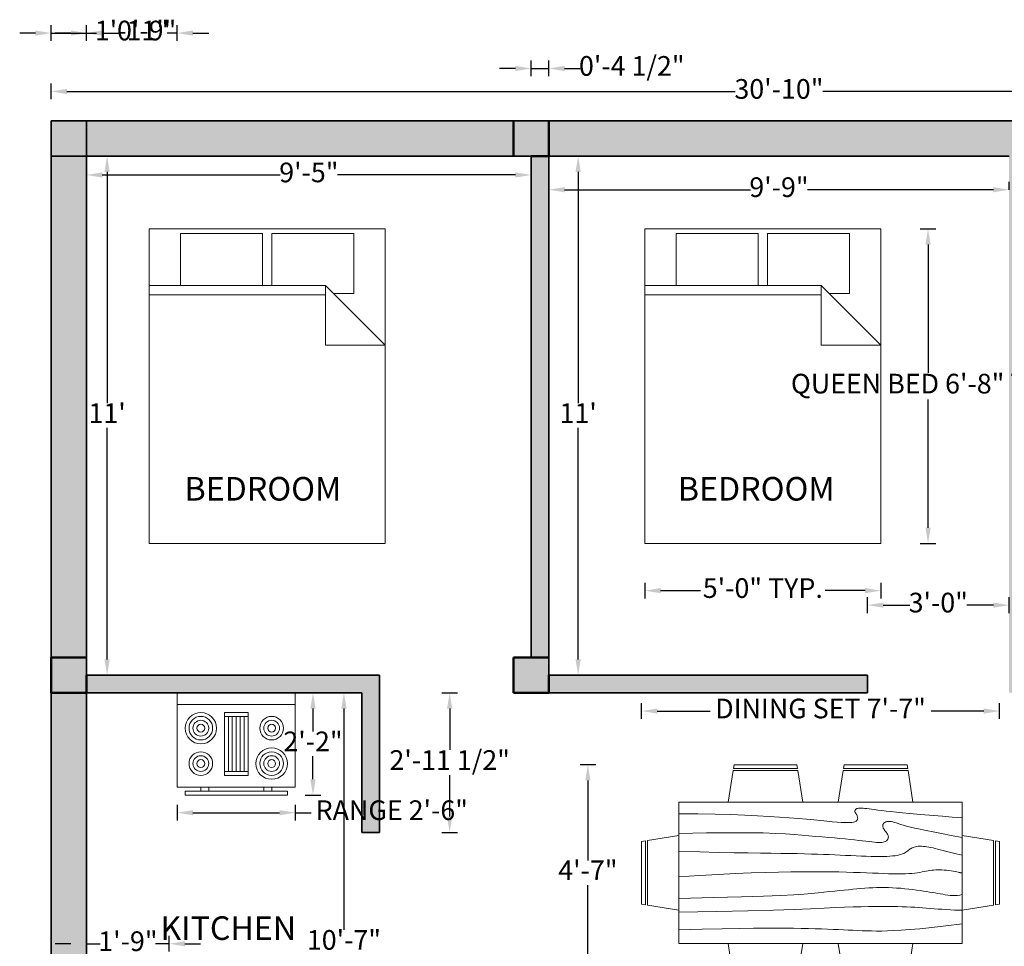
# Model space of a CAD drawing. Units: inches. Extents: x 2244 to 2676, y 593 to 1067.
# Tile 3 of 4: x 2268 to 2518, y 831 to 1067. Entities that reach past the tile are written whole.
import ezdxf

# ---------------------------------------------------------------- set-up
doc = ezdxf.new("R2010")
doc.units = ezdxf.units.IN
for name, color, linetype, lineweight in [('A-ANNO-DIMS', 2, 'Continuous', 18), ('A-AREA-IDEN', 7, 'Continuous', 25), ('A-COLS', 7, 'Continuous', 50), ('A-COLS-PATT', 1, 'Continuous', 13), ('A-EQPM', 8, 'Continuous', 18), ('A-FURN', 8, 'Continuous', 18), ('A-WALL', 7, 'Continuous', 35)]:
    doc.layers.add(name, color=color, linetype=linetype, lineweight=lineweight)
doc.layers.add('A-WALL-PATT', color=159, linetype='Continuous', lineweight=13, true_color=0x22346e)
doc.styles.get("Standard").update_dxf_attribs({"font": 'arial.ttf'})
doc.dimstyles.new('ISO-25', dxfattribs={"dimtxt": 5, "dimasz": 4, "dimexe": 2, "dimexo": 2, "dimtad": 0, "dimtih": 1, "dimtoh": 1, "dimlunit": 3, "dimtxsty": 'Standard', "dimcen": 2.5, "dimadec": 0, "dimazin": 0, "dimtfac": 1, "dimtmove": 0, "dimatfit": 3, "dimfxl": 2, "dimfxlon": 1, "dimarcsym": 0})

# ---------------------------------------------------------------- blocks, each defined once
blk = doc.blocks.new('*D4')
at = {"layer": 'A-ANNO-DIMS', "color": 0, "lineweight": -2, "transparency": 16777216}
for p, q in [((2288.42, 1031.92), (2292.42, 1031.92)), ((2290.42, 1027.92), (2290.42, 969.06)), ((2290.42, 903.92), (2290.42, 962.79)), ((2288.42, 899.92), (2292.42, 899.92))]:
    blk.add_line(p, q, dxfattribs=at)
at = {"layer": 'A-ANNO-DIMS', "color": 0, "transparency": 16777216}
for points in [[(2289.75, 1027.92), (2291.08, 1027.92), (2290.42, 1031.92)], [(2289.75, 903.92), (2291.08, 903.92), (2290.42, 899.92)]]:
    blk.add_solid(points, dxfattribs=at)
at = {"layer": 'Defpoints', "color": 0, "transparency": 16777216}
for p in [(2285.2, 1031.92), (2285.2, 899.92), (2290.42, 899.92)]:
    blk.add_point(p, dxfattribs=at)
at = {"layer": 'A-ANNO-DIMS', "color": 0, "transparency": 16777216, "insert": (2290.42, 965.92), "char_height": 5, "attachment_point": 5}
blk.add_mtext("11'", dxfattribs=at)
blk = doc.blocks.new('*D5')
at = {"layer": 'A-ANNO-DIMS', "color": 0, "lineweight": -2, "transparency": 16777216}
for p, q in [((2285.2, 1025.13), (2285.2, 1029.13)), ((2398.2, 1025.13), (2398.2, 1029.13)), ((2289.2, 1027.13), (2334.43, 1027.13)), ((2394.2, 1027.13), (2348.97, 1027.13))]:
    blk.add_line(p, q, dxfattribs=at)
at = {"layer": 'A-ANNO-DIMS', "color": 0, "transparency": 16777216}
for points in [[(2289.2, 1027.8), (2289.2, 1026.47), (2285.2, 1027.13)], [(2394.2, 1027.8), (2394.2, 1026.47), (2398.2, 1027.13)]]:
    blk.add_solid(points, dxfattribs=at)
at = {"layer": 'Defpoints', "color": 0, "transparency": 16777216}
for p in [(2398.2, 1027.13), (2285.2, 1019.69), (2398.2, 1019.69)]:
    blk.add_point(p, dxfattribs=at)
at = {"layer": 'A-ANNO-DIMS', "color": 0, "transparency": 16777216, "insert": (2341.7, 1027.13), "char_height": 5, "attachment_point": 5}
blk.add_mtext('9\'-5"', dxfattribs=at)
blk = doc.blocks.new('*D6')
at = {"layer": 'A-ANNO-DIMS', "color": 0, "lineweight": -2, "transparency": 16777216}
for p, q in [((2402.7, 1023.38), (2402.7, 1025.38)), ((2519.7, 1023.38), (2519.7, 1025.38)), ((2406.7, 1023.38), (2453.93, 1023.38)), ((2515.7, 1023.38), (2468.47, 1023.38))]:
    blk.add_line(p, q, dxfattribs=at)
at = {"layer": 'A-ANNO-DIMS', "color": 0, "transparency": 16777216}
for points in [[(2406.7, 1024.05), (2406.7, 1022.72), (2402.7, 1023.38)], [(2515.7, 1024.05), (2515.7, 1022.72), (2519.7, 1023.38)]]:
    blk.add_solid(points, dxfattribs=at)
at = {"layer": 'Defpoints', "color": 0, "transparency": 16777216}
for p in [(2402.7, 1023.38), (2402.7, 1022.02), (2519.7, 1022.02)]:
    blk.add_point(p, dxfattribs=at)
at = {"layer": 'A-ANNO-DIMS', "color": 0, "transparency": 16777216, "insert": (2461.2, 1023.38), "char_height": 5, "attachment_point": 5}
blk.add_mtext('9\'-9"', dxfattribs=at)
blk = doc.blocks.new('*D7')
at = {"layer": 'A-ANNO-DIMS', "color": 0, "lineweight": -2, "transparency": 16777216}
for p, q in [((2412.16, 1031.92), (2408.16, 1031.92)), ((2410.16, 1027.92), (2410.16, 969.06)), ((2410.16, 903.92), (2410.16, 962.79)), ((2412.16, 899.92), (2408.16, 899.92))]:
    blk.add_line(p, q, dxfattribs=at)
at = {"layer": 'A-ANNO-DIMS', "color": 0, "transparency": 16777216}
for points in [[(2409.49, 1027.92), (2410.82, 1027.92), (2410.16, 1031.92)], [(2409.49, 903.92), (2410.82, 903.92), (2410.16, 899.92)]]:
    blk.add_solid(points, dxfattribs=at)
at = {"layer": 'Defpoints', "color": 0, "transparency": 16777216}
for p in [(2414.35, 1031.92), (2410.16, 899.92), (2414.35, 899.92)]:
    blk.add_point(p, dxfattribs=at)
at = {"layer": 'A-ANNO-DIMS', "color": 0, "transparency": 16777216, "insert": (2410.16, 965.92), "char_height": 5, "attachment_point": 5}
blk.add_mtext("11'", dxfattribs=at)
blk = doc.blocks.new('*D21')
at = {"layer": 'A-ANNO-DIMS', "color": 0, "lineweight": -2, "transparency": 16777216}
for p, q in [((2276.2, 1046.37), (2276.2, 1050.37)), ((2646.2, 1046.37), (2646.2, 1050.37)), ((2280.2, 1048.37), (2450.04, 1048.37)), ((2642.2, 1048.37), (2472.35, 1048.37))]:
    blk.add_line(p, q, dxfattribs=at)
at = {"layer": 'A-ANNO-DIMS', "color": 0, "transparency": 16777216}
for points in [[(2280.2, 1049.03), (2280.2, 1047.7), (2276.2, 1048.37)], [(2642.2, 1049.03), (2642.2, 1047.7), (2646.2, 1048.37)]]:
    blk.add_solid(points, dxfattribs=at)
at = {"layer": 'Defpoints', "color": 0, "transparency": 16777216}
for p in [(2646.2, 1048.37), (2276.2, 1040.92), (2646.2, 1040.92)]:
    blk.add_point(p, dxfattribs=at)
at = {"layer": 'A-ANNO-DIMS', "color": 0, "transparency": 16777216, "insert": (2461.2, 1048.37), "char_height": 5, "attachment_point": 5}
blk.add_mtext('30\'-10"', dxfattribs=at)
blk = doc.blocks.new('Dining Set - 36 x 72 in.')
for p, q in [((-22.2343, 26.00059), (-23.4847, 17.99762)), ((-22.2304, 26), (-5.7608, 26)), ((-22, 27.5), (-22.1562, 26.50042)), ((-5.8416, 26.5), (-22.1534, 26.5)), ((-22, 27.5), (-6, 27.5)), ((-5.8437, 26.49966), (-6, 27.5)), ((-4.5152, 17.99762), (-5.7655, 25.99926)), ((5.7657, 26.00059), (4.5153, 17.99762)), ((5.7696, 26), (22.2392, 26)), ((6, 27.5), (5.8438, 26.50042)), ((22.1584, 26.5), (5.8466, 26.5)), ((6, 27.5), (22, 27.5)), ((22.1563, 26.49966), (22, 27.5)), ((23.4848, 17.99762), (22.2345, 25.99926)), ((36, 18), (-36, 18)), ((-36, 18), (-36, -18)), ((36, -18), (36, 18)), ((-45.5, 8), (-44.5004, 8.15617)), ((-45.5, 8), (-45.5, -8)), ((-44.5, -8.15843), (-44.5, 8.15338)), ((-44.0006, 8.23428), (-35.9976, 9.48474)), ((-44, 8.23041), (-44, -8.23915)), ((44.0006, 8.23428), (35.9976, 9.48474)), ((44, 8.23041), (44, -8.23915)), ((44.5, -8.15843), (44.5, 8.15338)), ((45.5, 8), (44.5005, 8.15617)), ((45.5, 8), (45.5, -8)), ((-44.4997, -8.15631), (-45.5, -8)), ((-35.9976, -9.48476), (-43.9993, -8.2345)), ((35.9976, -9.48476), (43.9993, -8.2345)), ((44.4997, -8.15631), (45.5, -8)), ((-36, -18), (36, -18)), ((-22.2343, -26.0006), (-23.4847, -17.99762)), ((-4.5152, -17.99762), (-5.7655, -25.99928)), ((5.7657, -26.0006), (4.5153, -17.99762)), ((23.4848, -17.99762), (22.2345, -25.99928)), ((-22.2304, -26), (-5.7608, -26)), ((-22, -27.5), (-22.1562, -26.50044)), ((-5.8416, -26.5), (-22.1534, -26.5)), ((-22, -27.5), (-6, -27.5)), ((-5.8437, -26.49967), (-6, -27.5)), ((5.7696, -26), (22.2392, -26)), ((6, -27.5), (5.8438, -26.50044)), ((22.1584, -26.5), (5.8466, -26.5)), ((6, -27.5), (22, -27.5)), ((22.1563, -26.49967), (22, -27.5))]:
    blk.add_line(p, q)
for points in [[(-36, 15), (-31.1772, 14.97754), (-26.8079, 14.91406), (-22.8538, 14.81543), (-19.276, 14.6875), (-16.0362, 14.53613), (-13.0957, 14.36718), (-10.4159, 14.18652), (-7.9583, 14), (-5.6904, 13.81315), (-3.6035, 13.63021), (-1.6954, 13.45508), (0.0365, 13.29166), (1.5945, 13.14388), (2.9811, 13.01562), (4.1988, 12.9108), (5.25, 12.83333), (6.1393, 12.78613), (6.8802, 12.76823), (7.4883, 12.77767), (7.9792, 12.8125), (8.3685, 12.87077), (8.6719, 12.95052), (8.9049, 13.0498), (9.0833, 13.16666), (9.2205, 13.29899), (9.3216, 13.44401), (9.3895, 13.59879), (9.4271, 13.76041), (9.4373, 13.92594), (9.4232, 14.09245), (9.3875, 14.257), (9.3333, 14.41666), (9.2638, 14.56917), (9.1836, 14.71484), (9.0975, 14.85465), (9.0104, 14.98958), (8.9272, 15.1206), (8.8529, 15.2487), (8.7922, 15.37483), (8.75, 15.5), (8.7305, 15.62467), (8.7344, 15.74739), (8.7617, 15.86621), (8.8125, 15.97916), (8.8867, 16.08431), (8.9844, 16.17968), (9.1055, 16.26334), (9.25, 16.33333), (9.4189, 16.38802), (9.6172, 16.42708), (9.8506, 16.45052), (10.125, 16.45833), (10.4463, 16.45052), (10.8203, 16.42708), (11.2529, 16.38802), (11.75, 16.33333), (12.3184, 16.26318), (12.9694, 16.17838), (13.7151, 16.07991), (14.5677, 15.96875), (15.5395, 15.84586), (16.6426, 15.71224), (17.8893, 15.56884), (19.2917, 15.41666), (20.859, 15.25667), (22.5879, 15.08984), (24.4721, 14.91715), (26.5052, 14.73958), (28.6809, 14.5581), (30.9929, 14.3737), (33.4347, 14.18733), (36, 14)], [(-36, 10), (-28.9766, 10.14274), (-23.1725, 10.20442), (-18.4241, 10.19775), (-14.5677, 10.13541), (-11.4399, 10.03011), (-8.877, 9.89453), (-6.7154, 9.74137), (-4.7917, 9.58333), (-2.9698, 9.43082), (-1.2246, 9.28515), (0.4415, 9.14534), (2.026, 9.01041), (3.5266, 8.87939), (4.9408, 8.7513), (6.266, 8.62516), (7.5, 8.5), (8.6411, 8.37549), (9.6914, 8.2539), (10.6538, 8.13818), (11.5312, 8.03125), (12.3267, 7.93603), (13.043, 7.85547), (13.6831, 7.79248), (14.25, 7.75), (14.7471, 7.7303), (15.1797, 7.73307), (15.5537, 7.75732), (15.875, 7.80208), (16.1494, 7.86637), (16.3828, 7.94922), (16.5811, 8.04964), (16.75, 8.16666), (16.8944, 8.29915), (17.0143, 8.44531), (17.1089, 8.60319), (17.1771, 8.77083), (17.218, 8.94629), (17.2305, 9.1276), (17.2137, 9.31282), (17.1667, 9.5), (17.0895, 9.6875), (16.987, 9.875), (16.8649, 10.0625), (16.7292, 10.25), (16.5856, 10.4375), (16.4401, 10.625), (16.2985, 10.8125), (16.1667, 11), (16.05, 11.18733), (15.9518, 11.3737), (15.8752, 11.5581), (15.8229, 11.73958), (15.798, 11.91715), (15.8034, 12.08984), (15.842, 12.25667), (15.9167, 12.41666), (16.0295, 12.56836), (16.1784, 12.70833), (16.3605, 12.83268), (16.5729, 12.9375), (16.8127, 13.01888), (17.0768, 13.07291), (17.3625, 13.0957), (17.6667, 13.08333), (17.9894, 13.03312), (18.3418, 12.94726), (18.7382, 12.82918), (19.1927, 12.68229), (19.7195, 12.51001), (20.3327, 12.31575), (21.0465, 12.10294), (21.875, 11.875), (22.8357, 11.63354), (23.959, 11.37304), (25.2786, 11.08618), (26.8282, 10.76562), (28.6414, 10.40405), (30.752, 9.99414), (33.1936, 9.52856), (36, 9)], [(-36, 5.5), (-30.7157, 5.3348), (-26.069, 5.20963), (-21.9946, 5.11767), (-18.4271, 5.05208), (-15.3009, 5.00602), (-12.5508, 4.97265), (-10.1112, 4.94515), (-7.9167, 4.91666), (-5.909, 4.88167), (-4.0586, 4.83984), (-2.3429, 4.79215), (-0.7396, 4.73958), (0.7739, 4.6831), (2.22, 4.6237), (3.6213, 4.56233), (5, 4.5), (6.373, 4.43782), (7.7344, 4.3776), (9.0723, 4.32129), (10.375, 4.27083), (11.6309, 4.22819), (12.8281, 4.19531), (13.9551, 4.17415), (15, 4.16666), (15.954, 4.17448), (16.819, 4.19791), (17.6001, 4.23698), (18.3021, 4.29166), (18.9299, 4.36198), (19.4883, 4.44791), (19.9823, 4.54948), (20.4167, 4.66666), (20.7969, 4.79899), (21.1302, 4.94401), (21.4245, 5.09879), (21.6875, 5.26041), (21.9271, 5.42594), (22.1511, 5.59245), (22.3672, 5.757), (22.5834, 5.91666), (22.8065, 6.06868), (23.0404, 6.21093), (23.2879, 6.34147), (23.5521, 6.45833), (23.8358, 6.55957), (24.142, 6.64323), (24.4735, 6.70735), (24.8334, 6.75), (25.2235, 6.76969), (25.642, 6.76692), (26.0858, 6.74267), (26.5521, 6.69791), (27.0379, 6.63362), (27.5404, 6.55078), (28.0565, 6.45036), (28.5834, 6.33333), (29.1242, 6.19987), (29.7071, 6.04687), (30.3661, 5.87044), (31.1354, 5.66666), (32.0493, 5.43164), (33.142, 5.16146), (34.4475, 4.85221), (36, 4.5)], [(-36, -1), (-30.7915, -0.6591), (-26.0195, -0.38216), (-21.6519, -0.16284), (-17.6563, 0.00521), (-14.0005, 0.12833), (-10.6523, 0.21289), (-7.5796, 0.26522), (-4.75, 0.29166), (-2.134, 0.29793), (0.2878, 0.28711), (2.5317, 0.26163), (4.6146, 0.22396), (6.5529, 0.17651), (8.3633, 0.12174), (10.0623, 0.06209), (11.6667, 0), (13.1899, -0.06201), (14.6341, -0.1211), (15.9982, -0.17432), (17.2813, -0.21875), (18.4823, -0.25147), (19.6003, -0.26953), (20.6343, -0.27002), (21.5834, -0.25), (22.4481, -0.20768), (23.2357, -0.14584), (23.9549, -0.06836), (24.6146, 0.02083), (25.2235, 0.11784), (25.7904, 0.21875), (26.3241, 0.31966), (26.8334, 0.41666), (27.3265, 0.50618), (27.8099, 0.58593), (28.2894, 0.65397), (28.7709, 0.70833), (29.2601, 0.74707), (29.763, 0.76823), (30.2855, 0.76985), (30.8334, 0.75), (31.4088, 0.70784), (31.9994, 0.64713), (32.589, 0.57275), (33.1615, 0.48958), (33.7008, 0.4025), (34.1908, 0.3164), (34.6153, 0.23616), (34.9584, 0.16666), (35.2099, 0.11165), (35.3848, 0.07031), (35.504, 0.04069), (35.5886, 0.02083), (35.6594, 0.00879), (35.7377, 0.0026), (35.8442, 0.00032), (36, 0)], [(-36, -6.5), (-27.1843, -6.31267), (-20.084, -6.1263), (-14.469, -5.9419), (-10.1094, -5.76042), (-6.7752, -5.58285), (-4.2363, -5.41016), (-2.2629, -5.24333), (-0.625, -5.08334), (0.8708, -4.93099), (2.2715, -4.78646), (3.5872, -4.64974), (4.8281, -4.52084), (6.0046, -4.39974), (7.127, -4.28646), (8.2053, -4.18099), (9.25, -4.08334), (10.2705, -3.99382), (11.2734, -3.91407), (12.2647, -3.84603), (13.25, -3.79167), (14.2354, -3.75293), (15.2266, -3.73177), (16.2295, -3.73015), (17.25, -3.75), (18.2912, -3.79248), (19.3451, -3.85547), (20.4009, -3.93604), (21.4479, -4.03125), (22.4754, -4.13819), (23.4727, -4.25391), (24.4289, -4.37549), (25.3334, -4.5), (26.1785, -4.62492), (26.9694, -4.74935), (27.7145, -4.87281), (28.4219, -4.99479), (29.1, -5.11483), (29.7572, -5.23242), (30.4016, -5.34709), (31.0417, -5.45834), (31.6837, -5.56437), (32.3262, -5.65821), (32.9658, -5.73153), (33.599, -5.77604), (34.2224, -5.78345), (34.8327, -5.74545), (35.4264, -5.65373), (36, -5.5)], [(-36, -10), (-26.4022, -9.81299), (-18.4675, -9.62891), (-11.9839, -9.45069), (-6.7396, -9.28125), (-2.5226, -9.12354), (0.8789, -8.98047), (3.6769, -8.85498), (6.0833, -8.75), (8.2767, -8.66765), (10.3021, -8.60677), (12.1712, -8.56543), (13.8958, -8.54167), (15.4876, -8.53353), (16.9583, -8.53907), (18.3197, -8.55632), (19.5834, -8.58334), (20.7616, -8.61841), (21.8685, -8.66081), (22.9188, -8.71004), (23.9271, -8.76563), (24.9081, -8.82707), (25.8763, -8.89388), (26.8465, -8.96558), (27.8334, -9.04167), (28.8474, -9.12118), (29.8828, -9.20117), (30.93, -9.27824), (31.9792, -9.34896), (33.0205, -9.40991), (34.0443, -9.45768), (35.0407, -9.48885), (36, -9.5)], [(-36, -14.5), (-30.0881, -14.33513), (-25.0332, -14.21224), (-20.7312, -14.12647), (-17.0781, -14.07292), (-13.97, -14.04671), (-11.3027, -14.04297), (-8.9724, -14.05681), (-6.875, -14.08334), (-4.9224, -14.11833), (-3.0905, -14.16016), (-1.3709, -14.20785), (0.2448, -14.26042), (1.7647, -14.3169), (3.1973, -14.3763), (4.5507, -14.43767), (5.8333, -14.5), (7.0554, -14.5621), (8.235, -14.62175), (9.3922, -14.67652), (10.5469, -14.72396), (11.7192, -14.76164), (12.929, -14.78711), (14.1965, -14.79794), (15.5417, -14.79167), (16.9933, -14.76424), (18.6152, -14.70508), (20.4804, -14.60197), (22.6615, -14.44271), (25.2312, -14.21509), (28.2624, -13.9069), (31.8277, -13.50594), (36, -13)]]:
    blk.add_lwpolyline(points)
blk = doc.blocks.new('Range-Oven - 30 in top')
for p, q in [((0, -3), (30, -3)), ((12, -6), (18, -6)), ((13, -20), (13, -6)), ((14, -6), (14, -20)), ((15, -20), (15, -6)), ((16, -6), (16, -20)), ((17, -20), (17, -6)), ((18, -20), (12, -20)), ((6, -24), (6, -25)), ((8, -25), (8, -24)), ((22, -25), (22, -24)), ((24, -24), (24, -25))]:
    blk.add_line(p, q)
for points in [[(0, -24), (0, 0), (30, 0), (30, -24)], [(12, -21), (12, -5), (18, -5), (18, -21)], [(2, -26), (2, -25), (28, -25), (28, -26)]]:
    blk.add_lwpolyline(points, close=True)
for centre, radius in [((6, -9), 4), ((6, -9), 3), ((6, -9), 2), ((24, -9), 3), ((24, -9), 2), ((6, -9), 1), ((24, -9), 1), ((6, -18), 3), ((24, -18), 4), ((24, -18), 3), ((6, -18), 2), ((6, -18), 1), ((24, -18), 2), ((24, -18), 1)]:
    blk.add_circle(centre, radius)
blk = doc.blocks.new('Bed - Queen')
for p, q in [((0, -80.00003), (0, 0)), ((0, 0), (59.99999, 0)), ((59.99999, 0), (59.99999, -80.00003)), ((7.99999, -1.2), (28.79998, -1.2)), ((7.99999, -14.4), (7.99999, -1.2)), ((28.79998, -1.2), (28.79998, -14.4)), ((31.19999, -1.2), (51.99999, -1.2)), ((31.19999, -14.4), (31.19999, -1.2)), ((51.99999, -1.2), (51.99999, -16.4)), ((0, -14.4), (44.8, -14.4)), ((59.99999, -29.6), (44.8, -14.4)), ((44.8, -14.4), (44.8, -29.6)), ((44.8, -16.8), (0, -16.8)), ((51.99999, -16.4), (46.79936, -16.4)), ((44.8, -29.6), (59.99999, -29.6)), ((59.99999, -80.00003), (0, -80.00003))]:
    blk.add_line(p, q)
blk = doc.blocks.new('*D28')
at = {"layer": 'A-ANNO-DIMS', "color": 0, "lineweight": -2, "transparency": 16777216}
for p, q in [((2352.62, 895.42), (2348.62, 895.42)), ((2350.62, 891.42), (2350.62, 835.1)), ((2350.62, 772.42), (2350.62, 828.74)), ((2352.62, 768.42), (2348.62, 768.42))]:
    blk.add_line(p, q, dxfattribs=at)
at = {"layer": 'A-ANNO-DIMS', "color": 0, "transparency": 16777216}
for points in [[(2349.96, 891.42), (2351.29, 891.42), (2350.62, 895.42)], [(2349.96, 772.42), (2351.29, 772.42), (2350.62, 768.42)]]:
    blk.add_solid(points, dxfattribs=at)
at = {"layer": 'Defpoints', "color": 0, "transparency": 16777216}
for p in [(2355.2, 895.42), (2350.62, 768.42), (2355.2, 768.42)]:
    blk.add_point(p, dxfattribs=at)
at = {"layer": 'A-ANNO-DIMS', "color": 0, "transparency": 16777216, "insert": (2350.62, 831.92), "char_height": 5, "attachment_point": 5}
blk.add_mtext('10\'-7"', dxfattribs=at)
blk = doc.blocks.new('*D30')
at = {"layer": 'A-ANNO-DIMS', "color": 0, "lineweight": -2, "transparency": 16777216}
for p, q in [((2497.1, 1013.41), (2501.1, 1013.41)), ((2499.1, 1009.41), (2499.1, 976.77)), ((2499.1, 937.41), (2499.1, 970.04)), ((2497.1, 933.41), (2501.1, 933.41))]:
    blk.add_line(p, q, dxfattribs=at)
at = {"layer": 'A-ANNO-DIMS', "color": 0, "transparency": 16777216}
for points in [[(2498.44, 1009.41), (2499.77, 1009.41), (2499.1, 1013.41)], [(2498.44, 937.41), (2499.77, 937.41), (2499.1, 933.41)]]:
    blk.add_solid(points, dxfattribs=at)
at = {"layer": 'Defpoints', "color": 0, "transparency": 16777216}
for p in [(2487.1, 1013.41), (2499.1, 1013.41), (2487.1, 933.41)]:
    blk.add_point(p, dxfattribs=at)
at = {"layer": 'A-ANNO-DIMS', "color": 0, "transparency": 16777216, "insert": (2499.1, 973.41), "char_height": 5, "attachment_point": 5}
blk.add_mtext('QUEEN BED 6\'-8" TYP.', dxfattribs=at)
blk = doc.blocks.new('*D31')
at = {"layer": 'A-ANNO-DIMS', "color": 0, "lineweight": -2, "transparency": 16777216}
for p, q in [((2427.1, 923.41), (2427.1, 919.41)), ((2431.1, 921.41), (2441.24, 921.41)), ((2483.1, 921.41), (2472.97, 921.41)), ((2487.1, 923.41), (2487.1, 919.41))]:
    blk.add_line(p, q, dxfattribs=at)
at = {"layer": 'A-ANNO-DIMS', "color": 0, "transparency": 16777216}
for points in [[(2431.1, 922.07), (2431.1, 920.74), (2427.1, 921.41)], [(2483.1, 922.07), (2483.1, 920.74), (2487.1, 921.41)]]:
    blk.add_solid(points, dxfattribs=at)
at = {"layer": 'Defpoints', "color": 0, "transparency": 16777216}
for p in [(2427.1, 933.41), (2487.1, 933.41), (2487.1, 921.41)]:
    blk.add_point(p, dxfattribs=at)
at = {"layer": 'A-ANNO-DIMS', "color": 0, "transparency": 16777216, "insert": (2457.1, 921.41), "char_height": 5, "attachment_point": 5}
blk.add_mtext('5\'-0" TYP.', dxfattribs=at)
blk = doc.blocks.new('*D32')
at = {"layer": 'A-ANNO-DIMS', "color": 0, "lineweight": -2, "transparency": 16777216}
for p, q in [((2426.28, 888.78), (2426.28, 892.78)), ((2517.28, 888.78), (2517.28, 892.78)), ((2430.28, 890.78), (2443.68, 890.78)), ((2513.28, 890.78), (2499.88, 890.78))]:
    blk.add_line(p, q, dxfattribs=at)
at = {"layer": 'A-ANNO-DIMS', "color": 0, "transparency": 16777216}
for points in [[(2430.28, 891.45), (2430.28, 890.11), (2426.28, 890.78)], [(2513.28, 891.45), (2513.28, 890.11), (2517.28, 890.78)]]:
    blk.add_solid(points, dxfattribs=at)
at = {"layer": 'Defpoints', "color": 0, "transparency": 16777216}
for p in [(2517.28, 890.78), (2426.28, 877.13), (2517.28, 877.13)]:
    blk.add_point(p, dxfattribs=at)
at = {"layer": 'A-ANNO-DIMS', "color": 0, "transparency": 16777216, "insert": (2471.78, 890.78), "char_height": 5, "attachment_point": 5}
blk.add_mtext('DINING SET 7\'-7"', dxfattribs=at)
blk = doc.blocks.new('*D33')
at = {"layer": 'A-ANNO-DIMS', "color": 0, "lineweight": -2, "transparency": 16777216}
for p, q in [((2414.63, 877.13), (2410.63, 877.13)), ((2412.63, 873.13), (2412.63, 852.75)), ((2412.63, 826.13), (2412.63, 846.5)), ((2414.63, 822.13), (2410.63, 822.13))]:
    blk.add_line(p, q, dxfattribs=at)
at = {"layer": 'A-ANNO-DIMS', "color": 0, "transparency": 16777216}
for points in [[(2411.96, 873.13), (2413.3, 873.13), (2412.63, 877.13)], [(2411.96, 826.13), (2413.3, 826.13), (2412.63, 822.13)]]:
    blk.add_solid(points, dxfattribs=at)
at = {"layer": 'Defpoints', "color": 0, "transparency": 16777216}
for p in [(2412.63, 877.13), (2426.28, 877.13), (2426.28, 822.13)]:
    blk.add_point(p, dxfattribs=at)
at = {"layer": 'A-ANNO-DIMS', "color": 0, "transparency": 16777216, "insert": (2412.63, 849.63), "char_height": 5, "attachment_point": 5}
blk.add_mtext('4\'-7"', dxfattribs=at)
blk = doc.blocks.new('*D37')
at = {"layer": 'A-ANNO-DIMS', "color": 0, "lineweight": -2, "transparency": 16777216}
for p, q in [((2285.2, 829.59), (2285.2, 833.59)), ((2306.2, 829.59), (2306.2, 833.59)), ((2281.2, 831.59), (2277.2, 831.59)), ((2285.2, 831.59), (2288.66, 831.59)), ((2306.2, 831.59), (2302.73, 831.59)), ((2310.2, 831.59), (2314.2, 831.59))]:
    blk.add_line(p, q, dxfattribs=at)
at = {"layer": 'A-ANNO-DIMS', "color": 0, "transparency": 16777216}
for points in [[(2281.2, 832.25), (2281.2, 830.92), (2285.2, 831.59)], [(2310.2, 832.25), (2310.2, 830.92), (2306.2, 831.59)]]:
    blk.add_solid(points, dxfattribs=at)
at = {"layer": 'Defpoints', "color": 0, "transparency": 16777216}
for p in [(2285.2, 831.59), (2285.2, 826.19), (2306.2, 826.19)]:
    blk.add_point(p, dxfattribs=at)
at = {"layer": 'A-ANNO-DIMS', "color": 0, "transparency": 16777216, "insert": (2295.7, 831.59), "char_height": 5, "attachment_point": 5}
blk.add_mtext('1\'-9"', dxfattribs=at)
blk = doc.blocks.new('*D38')
at = {"layer": 'A-ANNO-DIMS', "color": 0, "lineweight": -2, "transparency": 16777216}
for p, q in [((2308.25, 866.92), (2308.25, 862.92)), ((2338.25, 866.92), (2338.25, 862.92)), ((2312.25, 864.92), (2334.25, 864.92)), ((2338.25, 864.92), (2342.25, 864.92))]:
    blk.add_line(p, q, dxfattribs=at)
at = {"layer": 'A-ANNO-DIMS', "color": 0, "transparency": 16777216}
for points in [[(2312.25, 865.59), (2312.25, 864.25), (2308.25, 864.92)], [(2334.25, 865.59), (2334.25, 864.25), (2338.25, 864.92)]]:
    blk.add_solid(points, dxfattribs=at)
at = {"layer": 'Defpoints', "color": 0, "transparency": 16777216}
for p in [(2308.25, 869.42), (2338.25, 869.42), (2338.25, 864.92)]:
    blk.add_point(p, dxfattribs=at)
at = {"layer": 'A-ANNO-DIMS', "color": 0, "transparency": 16777216, "insert": (2362.78, 864.92), "char_height": 5, "attachment_point": 5}
blk.add_mtext('RANGE 2\'-6"', dxfattribs=at)
blk = doc.blocks.new('*D39')
at = {"layer": 'A-ANNO-DIMS', "color": 0, "lineweight": -2, "transparency": 16777216}
for p, q in [((2340.75, 895.42), (2344.75, 895.42)), ((2342.75, 891.42), (2342.75, 885.56)), ((2342.75, 873.42), (2342.75, 879.29)), ((2340.75, 869.42), (2344.75, 869.42))]:
    blk.add_line(p, q, dxfattribs=at)
at = {"layer": 'A-ANNO-DIMS', "color": 0, "transparency": 16777216}
for points in [[(2342.08, 891.42), (2343.42, 891.42), (2342.75, 895.42)], [(2342.08, 873.42), (2343.42, 873.42), (2342.75, 869.42)]]:
    blk.add_solid(points, dxfattribs=at)
at = {"layer": 'Defpoints', "color": 0, "transparency": 16777216}
for p in [(2338.25, 895.42), (2342.75, 895.42), (2338.25, 869.42)]:
    blk.add_point(p, dxfattribs=at)
at = {"layer": 'A-ANNO-DIMS', "color": 0, "transparency": 16777216, "insert": (2342.75, 882.42), "char_height": 5, "attachment_point": 5}
blk.add_mtext('2\'-2"', dxfattribs=at)
blk = doc.blocks.new('*D42')
at = {"layer": 'A-ANNO-DIMS', "color": 0, "lineweight": -2, "transparency": 16777216}
for p, q in [((2666.5, 859.92), (2670.5, 859.92)), ((2668.5, 855.92), (2668.5, 835.1)), ((2668.5, 807.92), (2668.5, 828.74)), ((2666.5, 803.92), (2670.5, 803.92))]:
    blk.add_line(p, q, dxfattribs=at)
at = {"layer": 'A-ANNO-DIMS', "color": 0, "transparency": 16777216}
for points in [[(2667.83, 855.92), (2669.16, 855.92), (2668.5, 859.92)], [(2667.83, 807.92), (2669.16, 807.92), (2668.5, 803.92)]]:
    blk.add_solid(points, dxfattribs=at)
at = {"layer": 'Defpoints', "color": 0, "transparency": 16777216}
for p in [(2359.7, 859.92), (2668.5, 859.92), (2359.7, 803.92)]:
    blk.add_point(p, dxfattribs=at)
at = {"layer": 'A-ANNO-DIMS', "color": 0, "transparency": 16777216, "insert": (2668.5, 831.92), "char_height": 5, "attachment_point": 5}
blk.add_mtext('4\'-8"', dxfattribs=at)
blk = doc.blocks.new('*D44')
at = {"layer": 'A-ANNO-DIMS', "color": 0, "lineweight": -2, "transparency": 16777216}
for p, q in [((2483.7, 915.72), (2483.7, 919.72)), ((2519.7, 915.72), (2519.7, 919.72)), ((2487.7, 917.72), (2494.43, 917.72)), ((2515.7, 917.72), (2508.97, 917.72))]:
    blk.add_line(p, q, dxfattribs=at)
at = {"layer": 'A-ANNO-DIMS', "color": 0, "transparency": 16777216}
for points in [[(2487.7, 918.39), (2487.7, 917.05), (2483.7, 917.72)], [(2515.7, 918.39), (2515.7, 917.05), (2519.7, 917.72)]]:
    blk.add_solid(points, dxfattribs=at)
at = {"layer": 'Defpoints', "color": 0, "transparency": 16777216}
for p in [(2519.7, 917.72), (2483.7, 895.42), (2519.7, 895.42)]:
    blk.add_point(p, dxfattribs=at)
at = {"layer": 'A-ANNO-DIMS', "color": 0, "transparency": 16777216, "insert": (2501.7, 917.72), "char_height": 5, "attachment_point": 5}
blk.add_mtext('3\'-0"', dxfattribs=at)
blk = doc.blocks.new('*D48')
at = {"layer": 'A-ANNO-DIMS', "color": 0, "lineweight": -2, "transparency": 16777216}
for p, q in [((2276.2, 1061.22), (2276.2, 1065.22)), ((2285.2, 1061.22), (2285.2, 1065.22)), ((2272.2, 1063.22), (2268.2, 1063.22)), ((2276.2, 1063.22), (2285.2, 1063.22)), ((2289.2, 1063.22), (2293.2, 1063.22))]:
    blk.add_line(p, q, dxfattribs=at)
at = {"layer": 'A-ANNO-DIMS', "color": 0, "transparency": 16777216}
for points in [[(2272.2, 1063.89), (2272.2, 1062.55), (2276.2, 1063.22)], [(2289.2, 1063.89), (2289.2, 1062.55), (2285.2, 1063.22)]]:
    blk.add_solid(points, dxfattribs=at)
at = {"layer": 'Defpoints', "color": 0, "transparency": 16777216}
for p in [(2285.2, 1063.22), (2276.2, 1040.92), (2285.2, 1040.92)]:
    blk.add_point(p, dxfattribs=at)
at = {"layer": 'A-ANNO-DIMS', "color": 0, "transparency": 16777216, "insert": (2300.47, 1063.22), "char_height": 5, "attachment_point": 5}
blk.add_mtext('0\'-9"', dxfattribs=at)
blk = doc.blocks.new('*D49')
at = {"layer": 'A-ANNO-DIMS', "color": 0, "lineweight": -2, "transparency": 16777216}
for p, q in [((2394.2, 1054.22), (2390.2, 1054.22)), ((2398.2, 1052.22), (2398.2, 1056.22)), ((2398.2, 1054.22), (2402.7, 1054.22)), ((2402.7, 1052.22), (2402.7, 1056.22)), ((2406.7, 1054.22), (2410.7, 1054.22))]:
    blk.add_line(p, q, dxfattribs=at)
at = {"layer": 'A-ANNO-DIMS', "color": 0, "transparency": 16777216}
for points in [[(2394.2, 1054.89), (2394.2, 1053.55), (2398.2, 1054.22)], [(2406.7, 1054.89), (2406.7, 1053.55), (2402.7, 1054.22)]]:
    blk.add_solid(points, dxfattribs=at)
at = {"layer": 'Defpoints', "color": 0, "transparency": 16777216}
for p in [(2402.7, 1054.22), (2398.2, 1031.92), (2402.7, 1031.92)]:
    blk.add_point(p, dxfattribs=at)
at = {"layer": 'A-ANNO-DIMS', "color": 0, "transparency": 16777216, "insert": (2423.79, 1054.22), "char_height": 5, "attachment_point": 5}
blk.add_mtext('0\'-4 1/2"', dxfattribs=at)
blk = doc.blocks.new('*D51')
at = {"layer": 'A-ANNO-DIMS', "color": 0, "lineweight": -2, "transparency": 16777216}
for p, q in [((2285.2, 1061.22), (2285.2, 1065.22)), ((2308.25, 1061.22), (2308.25, 1065.22)), ((2281.2, 1063.22), (2277.2, 1063.22)), ((2285.2, 1063.22), (2287.75, 1063.22)), ((2308.25, 1063.22), (2305.7, 1063.22)), ((2312.25, 1063.22), (2316.25, 1063.22))]:
    blk.add_line(p, q, dxfattribs=at)
at = {"layer": 'A-ANNO-DIMS', "color": 0, "transparency": 16777216}
for points in [[(2281.2, 1063.89), (2281.2, 1062.55), (2285.2, 1063.22)], [(2312.25, 1063.89), (2312.25, 1062.55), (2308.25, 1063.22)]]:
    blk.add_solid(points, dxfattribs=at)
at = {"layer": 'Defpoints', "color": 0, "transparency": 16777216}
for p in [(2308.25, 1063.22), (2285.2, 895.42), (2308.25, 895.42)]:
    blk.add_point(p, dxfattribs=at)
at = {"layer": 'A-ANNO-DIMS', "color": 0, "transparency": 16777216, "insert": (2296.72, 1063.22), "char_height": 5, "attachment_point": 5}
blk.add_mtext('1\'-11"', dxfattribs=at)
blk = doc.blocks.new('*D54')
at = {"layer": 'A-ANNO-DIMS', "color": 0, "lineweight": -2, "transparency": 16777216}
for p, q in [((2375.5, 895.42), (2379.5, 895.42)), ((2377.5, 891.42), (2377.5, 880.88)), ((2377.5, 863.92), (2377.5, 874.46)), ((2375.5, 859.92), (2379.5, 859.92))]:
    blk.add_line(p, q, dxfattribs=at)
at = {"layer": 'A-ANNO-DIMS', "color": 0, "transparency": 16777216}
for points in [[(2376.83, 891.42), (2378.16, 891.42), (2377.5, 895.42)], [(2376.83, 863.92), (2378.16, 863.92), (2377.5, 859.92)]]:
    blk.add_solid(points, dxfattribs=at)
at = {"layer": 'Defpoints', "color": 0, "transparency": 16777216}
for p in [(2355.2, 895.42), (2355.2, 859.92), (2377.5, 859.92)]:
    blk.add_point(p, dxfattribs=at)
at = {"layer": 'A-ANNO-DIMS', "color": 0, "transparency": 16777216, "insert": (2377.5, 877.67), "char_height": 5, "attachment_point": 5}
blk.add_mtext('2\'-11 1/2"', dxfattribs=at)

msp = doc.modelspace()

# ---------------------------------------------------------------- hatches: boundary and pattern name
at = {"layer": 'A-COLS-PATT'}
h = msp.add_hatch(color=256, dxfattribs=at)
h.dxf.hatch_style = 1
h.paths.add_polyline_path([(2285.197, 1040.922), (2276.197, 1040.922), (2276.197, 1031.922), (2285.197, 1031.922)])
h.paths.add_polyline_path([(2402.697, 1040.922), (2393.697, 1040.922), (2393.697, 1031.922), (2398.197, 1031.922), (2402.697, 1031.922)])
h.paths.add_polyline_path([(2528.697, 1040.922), (2519.697, 1040.922), (2519.697, 1031.922), (2524.197, 1031.922), (2528.697, 1031.922)])
h.paths.add_polyline_path([(2646.197, 1040.922), (2637.197, 1040.922), (2637.197, 1031.922), (2646.197, 1031.922)])
h.paths.add_polyline_path([(2646.197, 904.422), (2637.197, 904.422), (2637.197, 899.922), (2637.197, 895.422), (2646.197, 895.422)])
h.paths.add_polyline_path([(2528.697, 904.422), (2519.697, 904.422), (2519.697, 895.422), (2524.197, 895.422), (2528.697, 895.422)])
h.paths.add_polyline_path([(2402.697, 899.922), (2402.697, 904.422), (2393.697, 904.422), (2393.697, 895.422), (2402.697, 895.422)])
h.paths.add_polyline_path([(2285.197, 899.922), (2285.197, 904.422), (2276.197, 904.422), (2276.197, 895.422), (2285.197, 895.422)])
h.paths.add_polyline_path([(2285.197, 768.422), (2276.197, 768.422), (2276.197, 759.422), (2285.197, 759.422), (2285.197, 763.922)])
h.paths.add_polyline_path([(2285.197, 631.922), (2276.197, 631.922), (2276.197, 622.922), (2285.197, 622.922)])
h.paths.add_polyline_path([(2402.697, 631.922), (2398.197, 631.922), (2393.697, 631.922), (2393.697, 622.922), (2402.697, 622.922)])
h.paths.add_polyline_path([(2402.697, 763.922), (2402.697, 768.422), (2398.197, 768.422), (2393.697, 768.422), (2393.697, 759.422), (2402.697, 759.422)])
h.paths.add_polyline_path([(2528.697, 768.422), (2524.197, 768.422), (2519.697, 768.422), (2519.697, 759.422), (2528.697, 759.422)])
h.paths.add_polyline_path([(2528.697, 631.922), (2524.197, 631.922), (2519.697, 631.922), (2519.697, 628.922), (2519.697, 622.922), (2528.697, 622.922)])
h.paths.add_polyline_path([(2646.197, 631.922), (2637.197, 631.922), (2637.197, 622.922), (2646.197, 622.922)])
h.paths.add_polyline_path([(2646.197, 768.422), (2637.197, 768.422), (2637.197, 763.922), (2637.197, 759.422), (2646.197, 759.422)])
at = {"layer": 'A-WALL-PATT'}
h = msp.add_hatch(color=256, dxfattribs=at)
h.dxf.hatch_style = 1
h.paths.add_polyline_path([(2637.197, 1040.922), (2528.697, 1040.922), (2528.697, 1031.922), (2637.197, 1031.922)])
h.paths.add_polyline_path([(2519.697, 1040.922), (2402.697, 1040.922), (2402.697, 1031.922), (2519.697, 1031.922)])
h.paths.add_polyline_path([(2393.697, 1040.922), (2285.197, 1040.922), (2285.197, 1031.922), (2393.697, 1031.922)])
h.paths.add_polyline_path([(2285.197, 1031.922), (2276.197, 1031.922), (2276.197, 904.422), (2285.197, 904.422)])
h.paths.add_polyline_path([(2402.697, 1031.922), (2398.197, 1031.922), (2398.197, 904.422), (2402.697, 904.422)])
h.paths.add_polyline_path([(2483.697, 899.922), (2402.697, 899.922), (2402.697, 895.422), (2483.697, 895.422)])
h.paths.add_polyline_path([(2524.197, 1031.922), (2519.697, 1031.922), (2519.697, 904.422), (2524.197, 904.422)])
h.paths.add_polyline_path([(2637.197, 899.922), (2560.197, 899.922), (2560.197, 895.422), (2637.197, 895.422)])
h.paths.add_polyline_path([(2646.197, 1031.922), (2637.197, 1031.922), (2637.197, 904.422), (2646.197, 904.422)])
h.paths.add_polyline_path([(2646.197, 895.422), (2637.197, 895.422), (2637.197, 834.422), (2564.197, 834.422), (2564.197, 863.422), (2560.197, 863.422), (2560.197, 800.422), (2564.197, 800.422), (2564.197, 829.422), (2637.197, 829.422), (2637.197, 768.422), (2646.197, 768.422)])
h.paths.add_polyline_path([(2646.197, 759.422), (2637.197, 759.422), (2637.197, 631.922), (2646.197, 631.922)])
h.paths.add_polyline_path([(2637.197, 768.422), (2560.197, 768.422), (2560.197, 763.922), (2637.197, 763.922)])
h.paths.add_polyline_path([(2637.197, 631.922), (2528.697, 631.922), (2528.697, 622.922), (2637.197, 622.922)])
h.paths.add_polyline_path([(2524.197, 759.422), (2519.697, 759.422), (2519.697, 631.922), (2524.197, 631.922)])
h.paths.add_polyline_path([(2402.697, 759.422), (2398.197, 759.422), (2398.197, 631.922), (2402.697, 631.922)])
h.paths.add_polyline_path([(2476.697, 768.422), (2402.697, 768.422), (2402.697, 763.922), (2476.697, 763.922)])
h.paths.add_polyline_path([(2459.697, 631.922), (2402.697, 631.922), (2402.697, 622.922), (2459.697, 622.922), (2459.697, 628.922)])
h.paths.add_polyline_path([(2393.697, 631.922), (2285.197, 631.922), (2285.197, 622.922), (2393.697, 622.922)])
h.paths.add_polyline_path([(2285.197, 759.422), (2276.197, 759.422), (2276.197, 631.922), (2285.197, 631.922)])
h.paths.add_polyline_path([(2359.697, 803.922), (2355.197, 803.922), (2355.197, 768.422), (2285.197, 768.422), (2285.197, 763.922), (2359.697, 763.922)])
h.paths.add_polyline_path([(2359.697, 899.922), (2285.197, 899.922), (2285.197, 895.422), (2355.197, 895.422), (2355.197, 859.922), (2359.697, 859.922)])
h.paths.add_polyline_path([(2285.197, 895.422), (2276.197, 895.422), (2276.197, 768.422), (2285.197, 768.422)])

# ---------------------------------------------------------------- linework, layer by layer
at = {"layer": 'A-COLS'}
for p, q in [((2393.697, 1031.922), (2393.697, 1040.922)), ((2402.697, 1031.922), (2402.697, 1040.922)), ((2402.697, 1031.922), (2398.197, 1031.922)), ((2276.197, 895.422), (2276.197, 904.422)), ((2276.197, 904.422), (2285.197, 904.422)), ((2402.697, 904.422), (2393.697, 904.422)), ((2393.697, 904.422), (2393.697, 895.422)), ((2285.197, 899.922), (2285.197, 895.422)), ((2402.697, 895.422), (2402.697, 899.922)), ((2285.197, 895.422), (2276.197, 895.422)), ((2393.697, 895.422), (2402.697, 895.422))]:
    msp.add_line(p, q, dxfattribs=at)
at = {"layer": 'A-WALL'}
for p, q in [((2646.197, 1040.922), (2276.197, 1040.922)), ((2276.197, 1040.922), (2276.197, 622.922)), ((2285.197, 1040.922), (2285.197, 899.922)), ((2398.197, 1031.922), (2276.197, 1031.922)), ((2398.197, 1031.922), (2398.197, 904.422)), ((2402.697, 1031.922), (2402.697, 899.922)), ((2519.697, 1031.922), (2402.697, 1031.922)), ((2359.697, 899.922), (2285.197, 899.922)), ((2359.697, 899.922), (2359.697, 859.922)), ((2483.697, 899.922), (2402.697, 899.922)), ((2483.697, 899.922), (2483.697, 895.422)), ((2285.197, 895.422), (2285.197, 768.422)), ((2355.197, 895.422), (2285.197, 895.422)), ((2355.197, 895.422), (2355.197, 859.922)), ((2483.697, 895.422), (2398.197, 895.422)), ((2355.197, 859.922), (2359.697, 859.922))]:
    msp.add_line(p, q, dxfattribs=at)

# ---------------------------------------------------------------- block references
at = {"layer": 'A-EQPM'}
msp.add_blockref('Range-Oven - 30 in top', (2308.249, 895.422), dxfattribs=at)
at = {"layer": 'A-FURN'}
for name, p in [('Bed - Queen', (2301.112, 1013.405)), ('Bed - Queen', (2427.102, 1013.405)), ('Dining Set - 36 x 72 in.', (2471.779, 849.63))]:
    msp.add_blockref(name, p, dxfattribs=at)

# ---------------------------------------------------------------- texts
at = {"layer": 'A-AREA-IDEN', "char_height": 6, "attachment_point": 1}
for s, insert in [('BEDROOM', (2310.105, 950.313)), ('BEDROOM', (2435.513, 950.313)), ('KITCHEN', (2303.955, 838.569))]:
    msp.add_mtext_dynamic_manual_height_columns(s, width=31.51274, gutter_width=12.5, heights=[0], dxfattribs=dict(at, insert=insert))

# ---------------------------------------------------------------- dimensions: what is measured, and where the dimension line sits
at = {"layer": 'A-ANNO-DIMS'}
for base, p1, p2, override, picture, middle in [((2285.197, 1063.222), (2276.197, 1040.922), (2285.197, 1040.922), {"dimdec": 1, "dimlfac": 1, "dimrnd": 0, "dimzin": 1, "dimdsep": 46, "dimlunit": 4, "dimfrac": 2}, '*D48', (2300.467, 1063.222)), ((2308.249, 1063.222), (2285.197, 895.422), (2308.249, 895.422), {"dimdec": 1, "dimlfac": 1, "dimrnd": 0, "dimzin": 1, "dimdsep": 46, "dimlunit": 4, "dimfrac": 2}, '*D51', (2296.723, 1063.222)), ((2402.697, 1054.222), (2398.197, 1031.922), (2402.697, 1031.922), {"dimdec": 1, "dimlfac": 1, "dimrnd": 0, "dimzin": 1, "dimdsep": 46, "dimlunit": 4, "dimfrac": 2}, '*D49', (2423.793, 1054.222)), ((2646.197, 1048.367), (2276.197, 1040.922), (2646.197, 1040.922), {"dimclrd": 0, "dimclre": 0, "dimclrt": 0}, '*D21', (2461.197, 1048.367)), ((2398.197, 1027.135), (2285.197, 1019.689), (2398.197, 1019.689), {"dimclrd": 0, "dimclre": 0, "dimclrt": 0}, '*D5', (2341.697, 1027.135)), ((2402.697, 1023.385), (2519.697, 1022.016), (2402.697, 1022.016), {"dimclrd": 0, "dimclre": 0, "dimclrt": 0}, '*D6', (2461.197, 1023.385))]:
    dim = msp.add_linear_dim(base=base, p1=p1, p2=p2, dimstyle='ISO-25', override=override, dxfattribs=at)
    dim.commit()
    dim.dimension.update_dxf_attribs({"geometry": picture, "text_midpoint": middle})
for base, p1, p2, angle, override, picture, middle in [((2290.415, 899.922), (2285.197, 1031.922), (2285.197, 899.922), 90, {"dimclrd": 0, "dimclre": 0, "dimclrt": 0}, '*D4', (2290.415, 965.922)), ((2410.158, 899.922), (2414.351, 1031.922), (2414.351, 899.922), 90, {"dimclrd": 0, "dimclre": 0, "dimclrt": 0}, '*D7', (2410.158, 965.922)), ((2519.697, 917.722), (2483.697, 895.422), (2519.697, 895.422), 0, {"dimdec": 1, "dimlfac": 1, "dimrnd": 0, "dimzin": 1, "dimdsep": 46, "dimlunit": 4, "dimfrac": 2}, '*D44', (2501.697, 917.722)), ((2342.749, 895.422), (2338.249, 869.422), (2338.249, 895.422), 90, {"dimdec": 1, "dimlfac": 1, "dimrnd": 0, "dimzin": 1, "dimdsep": 46, "dimlunit": 4, "dimfrac": 2}, '*D39', (2342.749, 882.422)), ((2377.497, 859.922), (2355.197, 895.422), (2355.197, 859.922), 270, {"dimdec": 1, "dimlfac": 1, "dimrnd": 0, "dimzin": 1, "dimdsep": 46, "dimlunit": 4, "dimfrac": 2}, '*D54', (2377.497, 877.672)), ((2412.629, 877.13), (2426.279, 822.13), (2426.279, 877.13), 90, {"dimdec": 1, "dimlfac": 1, "dimrnd": 0, "dimzin": 1, "dimdsep": 46, "dimlunit": 4, "dimfrac": 2}, '*D33', (2412.629, 849.63)), ((2668.497, 859.922), (2359.697, 803.922), (2359.697, 859.922), 90, {"dimdec": 1, "dimlfac": 1, "dimrnd": 0, "dimzin": 1, "dimdsep": 46, "dimlunit": 4, "dimfrac": 2}, '*D42', (2668.497, 831.922)), ((2285.197, 831.585), (2306.197, 826.185), (2285.197, 826.185), 180, {"dimdec": 1, "dimlfac": 1, "dimrnd": 0, "dimzin": 1, "dimdsep": 46, "dimlunit": 4, "dimfrac": 2}, '*D37', (2295.697, 831.585))]:
    dim = msp.add_linear_dim(base=base, p1=p1, p2=p2, angle=angle, dimstyle='ISO-25', override=override, dxfattribs=at)
    dim.commit()
    dim.dimension.update_dxf_attribs({"geometry": picture, "text_midpoint": middle})
dim = msp.add_linear_dim(base=(2499.102, 1013.405), p1=(2487.102, 933.405), p2=(2487.102, 1013.405), angle=90, text='QUEEN BED <> TYP.', dimstyle='ISO-25', override={"dimdec": 1, "dimlfac": 1, "dimrnd": 0, "dimzin": 1, "dimdsep": 46, "dimlunit": 4, "dimfrac": 2}, dxfattribs=at)
dim.commit()
dim.dimension.update_dxf_attribs({"geometry": '*D30', "text_midpoint": (2499.102, 973.405)})
for base, p1, p2, text, picture, middle in [((2487.102, 921.405), (2427.102, 933.405), (2487.102, 933.405), '<> TYP.', '*D31', (2457.102, 921.405)), ((2517.279, 890.78), (2426.279, 877.13), (2517.279, 877.13), 'DINING SET <>', '*D32', (2471.779, 890.78)), ((2338.249, 864.922), (2308.249, 869.422), (2338.249, 869.422), 'RANGE <>', '*D38', (2362.781, 864.922))]:
    dim = msp.add_linear_dim(base=base, p1=p1, p2=p2, text=text, dimstyle='ISO-25', override={"dimdec": 1, "dimlfac": 1, "dimrnd": 0, "dimzin": 1, "dimdsep": 46, "dimlunit": 4, "dimfrac": 2}, dxfattribs=at)
    dim.commit()
    dim.dimension.update_dxf_attribs({"geometry": picture, "text_midpoint": middle})
dim = msp.add_linear_dim(base=(2350.624, 768.422), p1=(2355.197, 895.422), p2=(2355.197, 768.422), angle=90, dimstyle='ISO-25', override={"dimclrd": 0, "dimclre": 0, "dimclrt": 0}, dxfattribs=at)
dim.commit()
dim.dimension.update_dxf_attribs({"geometry": '*D28', "text_midpoint": (2350.624, 831.922), "dimtype": 160})

doc.saveas('drawing.dxf')
